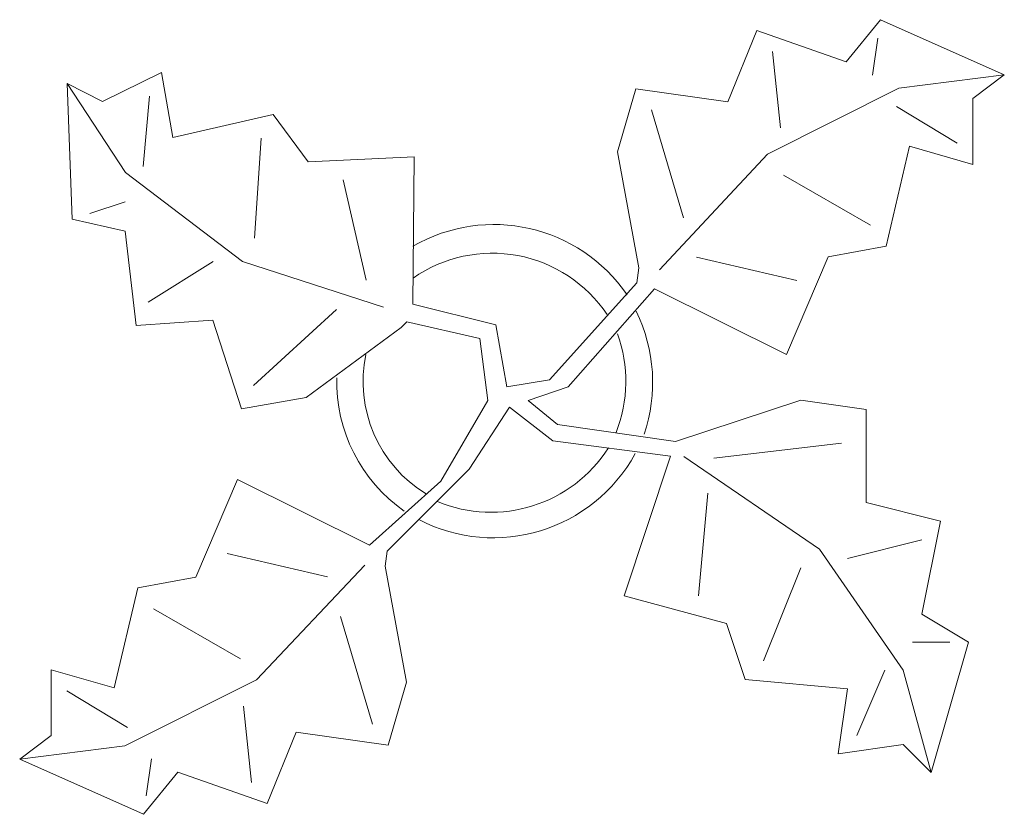
# Model space of a CAD drawing. Units: inches. Extents: x 13 to 1693, y -7 to 1519.
# Tile 10 of 10: x 1094 to 1132, y 1461 to 1491. Entities that reach past the tile are written whole.
import ezdxf

# ---------------------------------------------------------------- set-up
doc = ezdxf.new("R2010")
doc.units = ezdxf.units.IN
doc.header["$MEASUREMENT"] = 0
doc.layers.add('TREE', color=102, linetype='Continuous', lineweight=18)

# ---------------------------------------------------------------- blocks, each defined once
blk = doc.blocks.new('Plant - Rubber or Philodendron')
for p, q in [((13.3837, 12.301), (14.68, 13.9039)), ((14.68, 13.9039), (19.3848, 11.8146)), ((8.8871, 10.7908), (9.9809, 13.4933)), ((9.9809, 13.4933), (13.3837, 12.301)), ((14.5816, 13.2037), (14.3848, 11.8033)), ((10.5828, 12.6946), (10.8893, 9.7953)), ((-14.8639, 10.7964), (-12.6195, 11.8975)), ((-12.6195, 11.8975), (-12.1909, 9.4345)), ((19.3848, 11.8146), (15.3859, 11.3055)), ((19.3848, 11.8146), (18.1868, 10.9119)), ((-16.2005, 11.4774), (-13.9899, 8.1064)), ((-16.2005, 11.4774), (-14.8639, 10.7964)), ((-16.0159, 6.3329), (-16.2005, 11.4774)), ((4.6914, 8.8812), (5.3859, 11.2828)), ((5.3859, 11.2828), (8.8871, 10.7908)), ((15.3859, 11.3055), (10.3916, 8.7942)), ((-13.3174, 8.325), (-13.0735, 11.0065)), ((18.1868, 10.9119), (18.1925, 8.4119)), ((5.9878, 10.4842), (7.1971, 6.3869)), ((15.2875, 10.6053), (17.5907, 9.2105)), ((-12.1909, 9.4345), (-8.3829, 10.3)), ((-8.3829, 10.3), (-7.0549, 8.501)), ((-8.8369, 9.409), (-9.0894, 5.6095)), ((15.7909, 9.1065), (14.8995, 5.3044)), ((18.1925, 8.4119), (15.7909, 9.1065)), ((-7.0549, 8.501), (-3.0284, 8.6941)), ((-3.0284, 8.6941), (-3.0709, 3.1041)), ((4.6914, 8.8812), (5.5014, 4.4831)), ((10.3916, 8.7942), (6.2847, 4.4028)), ((-13.9899, 8.1064), (-9.5434, 4.7185)), ((14.2977, 6.1031), (10.9934, 7.9956)), ((-4.8529, 4.012), (-5.7184, 7.82)), ((-15.3434, 6.5514), (-13.9984, 6.9884)), ((-14.0069, 5.8704), (-16.0159, 6.3329)), ((-13.5868, 2.2894), (-14.0069, 5.8704)), ((14.8995, 5.3044), (12.7005, 4.8994)), ((7.7005, 4.8881), (11.5025, 3.9967)), ((12.7005, 4.8994), (11.1089, 1.1958)), ((-13.1329, 3.1804), (-10.6614, 4.727)), ((-9.5434, 4.7185), (-4.1917, 2.9888)), ((5.4346, 3.9146), (5.5014, 4.4831)), ((2.1141, 0.2298), (5.4346, 3.9146)), ((6.1032, 3.6844), (2.8262, -0.031)), ((11.1089, 1.1958), (6.1032, 3.6844)), ((-3.0709, 3.1041), (0.0797, 2.3163)), ((-9.1318, 0.0195), (-5.9793, 2.9025)), ((-10.6784, 2.491), (-13.5868, 2.2894)), ((-9.5858, -0.8715), (-10.6784, 2.491)), ((-3.5248, 2.2131), (-3.3011, 2.4355)), ((-3.3011, 2.4355), (-0.5306, 1.7947)), ((0.0797, 2.3163), (0.4866, -0.031)), ((-7.1228, -0.443), (-3.5248, 2.2131)), ((-0.5306, 1.7947), (-0.2255, -0.5527)), ((-0.5306, 1.7947), (-0.5306, 1.7947)), ((0.4866, -0.031), (2.1141, 0.2298)), ((2.8262, -0.031), (1.3003, -0.5527)), ((-7.1228, -0.443), (-9.5858, -0.8715)), ((-2.019, -3.6148), (-0.2255, -0.5527)), ((1.3003, -0.5527), (2.4193, -1.4655)), ((11.6605, -0.5413), (6.895, -2.1175)), ((11.6605, -0.5413), (14.1354, -0.8948)), ((-0.9375, -3.1608), (0.5883, -0.8135)), ((0.5883, -0.8135), (2.2447, -2.0916)), ((14.1354, -0.8948), (14.1354, -4.4304)), ((2.4193, -1.4655), (6.895, -2.1175)), ((2.2447, -2.0916), (6.7108, -2.6626)), ((8.3544, -2.7453), (13.1973, -2.1704)), ((4.943, -7.9659), (6.7108, -2.6626)), ((12.3677, -6.1981), (7.219, -2.6772)), ((-4.0579, -6.2781), (-0.9375, -3.1608)), ((-11.3237, -7.2629), (-9.7321, -3.5593)), ((-9.7321, -3.5593), (-4.7264, -6.0479)), ((-2.019, -3.6148), (-4.7264, -6.0479)), ((8.125, -4.0768), (7.7715, -7.9659)), ((14.1354, -4.4304), (16.9638, -5.1375)), ((16.9638, -5.1375), (16.2567, -8.673)), ((16.2567, -5.8446), (13.4283, -6.5517)), ((-4.1246, -6.8466), (-4.0579, -6.2781)), ((15.5496, -10.7943), (12.3677, -6.1981)), ((-6.3237, -7.2516), (-10.1257, -6.3602)), ((-9.0148, -11.1577), (-4.9047, -6.8122)), ((-3.3146, -11.2447), (-4.1246, -6.8466)), ((10.2463, -10.4408), (11.6605, -6.9053)), ((-13.5228, -7.6679), (-11.3237, -7.2629)), ((-14.4141, -11.4699), (-13.5228, -7.6679)), ((8.8321, -9.0266), (4.943, -7.9659)), ((-12.921, -8.4665), (-9.6166, -10.359)), ((-4.611, -12.8477), (-5.8203, -8.7504)), ((16.2567, -8.673), (18.0245, -9.7337)), ((9.5392, -11.1479), (8.8321, -9.0266)), ((17.3174, -9.7337), (15.9032, -9.7337)), ((18.0245, -9.7337), (16.6103, -14.6834)), ((-16.8157, -10.7754), (-14.4141, -11.4699)), ((-16.8101, -13.2754), (-16.8157, -10.7754)), ((14.8425, -10.7943), (13.7819, -13.2692)), ((16.6103, -14.6834), (15.5496, -10.7943)), ((-14.0091, -13.669), (-9.0148, -11.1577)), ((13.4283, -11.5015), (9.5392, -11.1479)), ((-13.9107, -12.9688), (-16.2139, -11.574)), ((-3.3146, -11.2447), (-4.0092, -13.6463)), ((13.0748, -13.9763), (13.4283, -11.5015)), ((-9.206, -15.0581), (-9.5126, -12.1588)), ((-18.008, -14.1781), (-16.8101, -13.2754)), ((-7.5103, -13.1543), (-8.6042, -15.8568)), ((-4.0092, -13.6463), (-7.5103, -13.1543)), ((-18.008, -14.1781), (-14.0091, -13.669)), ((15.5496, -13.6228), (13.0748, -13.9763)), ((16.6103, -14.6834), (15.5496, -13.6228)), ((-13.3032, -16.2674), (-18.008, -14.1781)), ((-13.2048, -15.5672), (-13.008, -14.1668)), ((-12.0069, -14.6645), (-13.3032, -16.2674)), ((-8.6042, -15.8568), (-12.0069, -14.6645))]:
    blk.add_line(p, q)
for centre, radius, start, end in [((0, 0), 6.1275, 34.37569, 120.1028), ((-0.0601, -0.2075), 5.2461, 33.82192, 124.9414), ((-0.098, 0.1364), 6.1288, 341.2017, 26.09184), ((-0.2664, 0.1682), 5.2775, 338.4094, 20.03007), ((0.0308, 0.1664), 5, 168.1647, 238.6725), ((0.0308, 0.1664), 6, 178.6147, 235.1169), ((-0.0234, 0.3825), 6.1492, 242.5812, 331.2714), ((-0.1102, 0.4886), 5.2883, 247.3711, 327.472)]:
    blk.add_arc(centre, radius, start, end)

msp = doc.modelspace()

# ---------------------------------------------------------------- block references
at = {"layer": 'TREE'}
msp.add_blockref('Plant - Rubber or Philodendron', (1112.119, 1477.035), dxfattribs=at)

doc.saveas('drawing.dxf')
